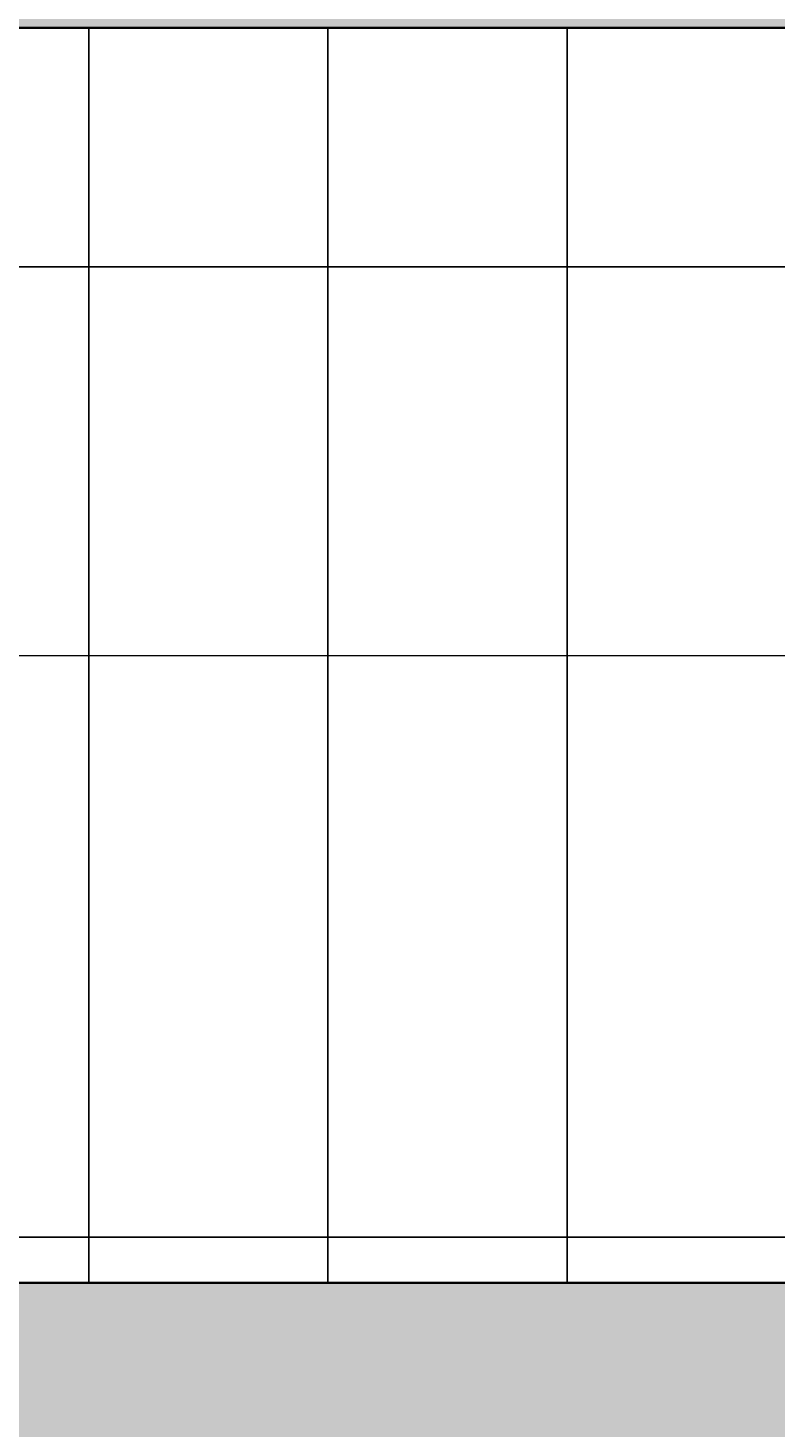
# Model space of a CAD drawing. Units: inches. Extents: x 1998 to 2588, y 1139 to 1977.
# Tile 107 of 134: x 2422 to 2447, y 1590 to 1637. Entities that reach past the tile are written whole.
import ezdxf

# ---------------------------------------------------------------- set-up
doc = ezdxf.new("R2010")
doc.units = ezdxf.units.IN
for name, color, linetype, lineweight in [('A-ANNO-DIMS', 2, 'Continuous', 18), ('A-ANNO-SYMB', 7, 'Continuous', 18), ('A-FLOR-EVTR', 7, 'Continuous', 35), ('A-FLOR-STRS', 7, 'Continuous', 25), ('A-WALL-PATT', 252, 'Continuous', 13), ('WALL', 200, 'Continuous', 35)]:
    doc.layers.add(name, color=color, linetype=linetype, lineweight=lineweight)
doc.styles.get("Standard").update_dxf_attribs({"font": 'arial.ttf'})
doc.dimstyles.get("Standard").update_dxf_attribs({"dimtxt": 0.18, "dimasz": 0.18, "dimexe": 0.18, "dimexo": 0.0625, "dimgap": 0.09, "dimtad": 0, "dimtih": 1, "dimtoh": 1, "dimdec": 4, "dimzin": 0, "dimdsep": 46, "dimtxsty": 'Standard', "dimcen": 0.09, "dimadec": 0, "dimazin": 0, "dimtfac": 1, "dimtdec": 4, "dimtofl": 0, "dimtmove": 0, "dimatfit": 3, "dimfxl": 1, "dimtolj": 1, "dimtzin": 0, "dimarcsym": 0})

# ---------------------------------------------------------------- blocks, each defined once
blk = doc.blocks.new('*D24')
at = {"layer": 'A-ANNO-DIMS', "color": 0, "lineweight": -2, "transparency": 16777216}
for p, q in [((2398.535, 1911.232), (2588.309, 1911.232)), ((2588.129, 1911.052), (2588.129, 1570.164)), ((2588.129, 1228.912), (2588.129, 1569.8)), ((2527.535, 1228.732), (2588.309, 1228.732))]:
    blk.add_line(p, q, dxfattribs=at)
at = {"layer": 'A-ANNO-DIMS', "color": 0, "transparency": 16777216}
for points in [[(2588.099, 1911.052), (2588.159, 1911.052), (2588.129, 1911.232)], [(2588.099, 1228.912), (2588.159, 1228.912), (2588.129, 1228.732)]]:
    blk.add_solid(points, dxfattribs=at)
at = {"layer": 'Defpoints', "color": 0, "transparency": 16777216}
for p in [(2398.473, 1911.232), (2588.129, 1911.232), (2527.473, 1228.732)]:
    blk.add_point(p, dxfattribs=at)
at = {"layer": 'A-ANNO-DIMS', "color": 0, "transparency": 16777216, "insert": (2588.129, 1569.982), "char_height": 0.18, "attachment_point": 5}
blk.add_mtext('\\A1;682.5', dxfattribs=at)
blk = doc.blocks.new('*D39')
at = {"layer": 'A-ANNO-DIMS', "color": 0, "lineweight": -2, "transparency": 16777216}
for p, q in [((2115.035, 1628.742), (2588.309, 1628.742)), ((2588.129, 1628.562), (2588.129, 1612.685)), ((2588.129, 1596.444), (2588.129, 1612.321)), ((2115.035, 1596.264), (2588.309, 1596.264))]:
    blk.add_line(p, q, dxfattribs=at)
at = {"layer": 'A-ANNO-DIMS', "color": 0, "transparency": 16777216}
for points in [[(2588.099, 1628.562), (2588.159, 1628.562), (2588.129, 1628.742)], [(2588.099, 1596.444), (2588.159, 1596.444), (2588.129, 1596.264)]]:
    blk.add_solid(points, dxfattribs=at)
at = {"layer": 'Defpoints', "color": 0, "transparency": 16777216}
for p in [(2114.973, 1628.742), (2588.129, 1628.742), (2114.973, 1596.264)]:
    blk.add_point(p, dxfattribs=at)
at = {"layer": 'A-ANNO-DIMS', "color": 0, "transparency": 16777216, "insert": (2588.129, 1612.503), "char_height": 0.18, "attachment_point": 5}
blk.add_mtext('\\A1;32.48', dxfattribs=at)

msp = doc.modelspace()

# ---------------------------------------------------------------- hatches: boundary and pattern name
at = {"layer": 'A-WALL-PATT'}
h = msp.add_hatch(color=256, dxfattribs=at)
h.dxf.hatch_style = 1
h.paths.add_polyline_path([(2527.4729, 1362.2324), (2510.9729, 1362.2324), (2510.9729, 1357.7324), (2518.4729, 1357.7324), (2518.4729, 1237.7324), (2503.1458, 1237.7324), (2503.1458, 1228.7324), (2527.4729, 1228.7324)])
h.paths.add_polyline_path([(2490.5682, 1362.2324), (2398.4729, 1362.2324), (2398.4729, 1357.7324), (2490.5682, 1357.7324)])
h.paths.add_polyline_path([(2224.9729, 1264.7324), (2222.9729, 1264.7324), (2222.9729, 1232.4125), (2341.4729, 1232.4125), (2341.4729, 1234.4125), (2224.9729, 1234.4125)])
h.paths.add_polyline_path([(2334.5332, 1273.7324), (2264.7638, 1273.7324), (2264.7638, 1269.5611, -0.043659), (2264.3413, 1264.7324), (2334.5332, 1264.7324)])
h.paths.add_polyline_path([(2236.9551, 1273.7324), (2234.4125, 1273.7324), (2234.4125, 1264.7324), (2236.9551, 1264.7324), (2236.9551, 1269.5611)])
h.paths.add_polyline_path([(2222.9729, 1293.2324), (2096.9729, 1293.2324), (2096.9729, 1345.0966), (2087.9729, 1345.0966), (2087.9729, 1284.2324), (2222.9729, 1284.2324), (2222.9729, 1285.137)])
h.paths.add_polyline_path([(2096.9729, 1458.7927), (2087.9729, 1458.7927), (2087.9729, 1417.7324), (2087.9729, 1413.2324), (2096.9729, 1413.2324), (2096.9729, 1417.7324)])
h.paths.add_polyline_path([(2096.9729, 1413.2324), (2087.9729, 1413.2324), (2087.9729, 1365.5012), (2096.9729, 1365.5012), (2096.9729, 1369.3358)])
h.paths.add_polyline_path([(2186.2943, 1417.7324), (2138.6074, 1417.7324), (2096.9729, 1417.7324), (2096.9729, 1413.2324), (2138.6074, 1413.2324), (2186.2943, 1413.2324)])
h.paths.add_polyline_path([(2181.4729, 1465.7324), (2176.9729, 1465.7324), (2176.9729, 1451.6434), (2181.4729, 1451.6434)])
h.paths.add_polyline_path([(2181.4729, 1422.1664), (2176.9729, 1422.1664), (2176.9729, 1417.7324), (2181.4729, 1417.7324)])
h.paths.add_polyline_path([(2063.9729, 1465.7324), (2087.9729, 1465.7324), (2087.9729, 1470.2324), (2059.4729, 1470.2324), (2059.4729, 1413.2324), (2087.9729, 1413.2324), (2087.9729, 1417.7324), (2063.9729, 1417.7324)])
h.paths.add_polyline_path([(2181.4729, 1755.2324), (2176.9729, 1755.2324), (2176.9729, 1748.6798), (2177.0513, 1748.6798), (2181.4729, 1748.6798)])
h.paths.add_polyline_path([(2227.4729, 1707.2324), (2220.4647, 1707.2324), (2220.4647, 1702.7324), (2222.9729, 1702.7324), (2222.9729, 1604.637), (2227.4729, 1604.637)])
h.paths.add_polyline_path([(2114.9729, 1702.7324), (2105.9729, 1702.7324), (2105.9729, 1628.4781, -0.0318759), (2110.1012, 1628.7416), (2114.9729, 1628.7416)])
h.paths.add_polyline_path([(2345.9729, 1739.3278), (2341.4729, 1739.3278), (2341.4729, 1647.5211), (2345.9729, 1647.5211)])
h.paths.add_polyline_path([(2350.6273, 1641.2324), (2345.9729, 1641.2324), (2345.9729, 1636.7324), (2350.6273, 1636.7324), (2350.6273, 1639.8729)])
h.paths.add_polyline_path([(2501.9729, 1641.2324), (2407.9729, 1641.2324), (2392.5005, 1641.2324), (2392.5005, 1639.8729), (2392.5005, 1636.7324), (2501.9729, 1636.7324)])
h.paths.add_polyline_path([(2510.9729, 1755.2324), (2501.9729, 1755.2324), (2501.9729, 1641.2324), (2510.9729, 1641.2324)])
h.paths.add_polyline_path([(2549.1786, 1641.2324), (2522.3775, 1641.2324), (2522.3775, 1636.7324), (2540.1786, 1636.7324), (2540.1786, 1480.7324), (2522.3775, 1480.7324), (2522.3775, 1476.2324), (2549.1786, 1476.2324)])
h.paths.add_polyline_path([(2498.1786, 1594.7324), (2407.9729, 1594.7324), (2407.9729, 1585.7324), (2416.9729, 1585.7324), (2489.1786, 1585.7324), (2489.1786, 1531.7324), (2416.9729, 1531.7324), (2407.9729, 1531.7324), (2407.9729, 1522.7324), (2498.1786, 1522.7324)])
h.paths.add_polyline_path([(2351.6437, 1480.7324), (2345.9729, 1480.7324), (2345.9729, 1476.2324), (2351.6437, 1476.2324), (2351.6437, 1477.5919)])
h.paths.add_polyline_path([(2501.9729, 1480.7324), (2498.1786, 1480.7324), (2407.9729, 1480.7324), (2393.5168, 1480.7324), (2393.5168, 1477.5919), (2393.5168, 1476.2324), (2501.9729, 1476.2324)])

# ---------------------------------------------------------------- linework, layer by layer
at = {"layer": 'A-ANNO-SYMB'}
msp.add_line((2407.9729, 1615.7324), (2505.7676, 1615.7324), dxfattribs=at)
at = {"layer": 'A-FLOR-EVTR'}
msp.add_lwpolyline([(2407.9729, 1522.7324), (2498.1786, 1522.7324), (2498.1786, 1594.7324), (2407.9729, 1594.7324)], close=True, dxfattribs=at)
at = {"layer": 'A-FLOR-STRS'}
for p, q in [((2423.9729, 1636.7324), (2423.9729, 1594.7324)), ((2431.9729, 1636.7324), (2431.9729, 1594.7324)), ((2439.9729, 1636.7324), (2439.9729, 1594.7324)), ((2407.9729, 1594.7324), (2540.1786, 1594.7324))]:
    msp.add_line(p, q, dxfattribs=at)
at = {"layer": 'WALL'}
for p, q in [((2501.9729, 1636.7324), (2392.5005, 1636.7324)), ((2407.9729, 1636.7324), (2501.9729, 1636.7324))]:
    msp.add_line(p, q, dxfattribs=at)

# ---------------------------------------------------------------- dimensions: what is measured, and where the dimension line sits
at = {"layer": 'A-ANNO-DIMS'}
for base, p1, p2, override, picture, middle in [((2588.1286, 1911.2324), (2527.4729, 1228.7324), (2398.4729, 1911.2324), {"dimdec": 1, "dimlfac": 1, "dimrnd": 0, "dimzin": 0, "dimdsep": 46, "dimlunit": 2}, '*D24', (2588.1286, 1569.9824)), ((2588.1286, 1628.7416), (2114.9729, 1596.2642), (2114.9729, 1628.7416), {"dimdec": 2, "dimlfac": 1, "dimrnd": 0, "dimzin": 0, "dimdsep": 46, "dimlunit": 2}, '*D39', (2588.1286, 1612.5029))]:
    dim = msp.add_linear_dim(base=base, p1=p1, p2=p2, angle=90, dimstyle='Standard', override=override, dxfattribs=at)
    dim.commit()
    dim.dimension.update_dxf_attribs({"geometry": picture, "text_midpoint": middle})

doc.saveas('drawing.dxf')
